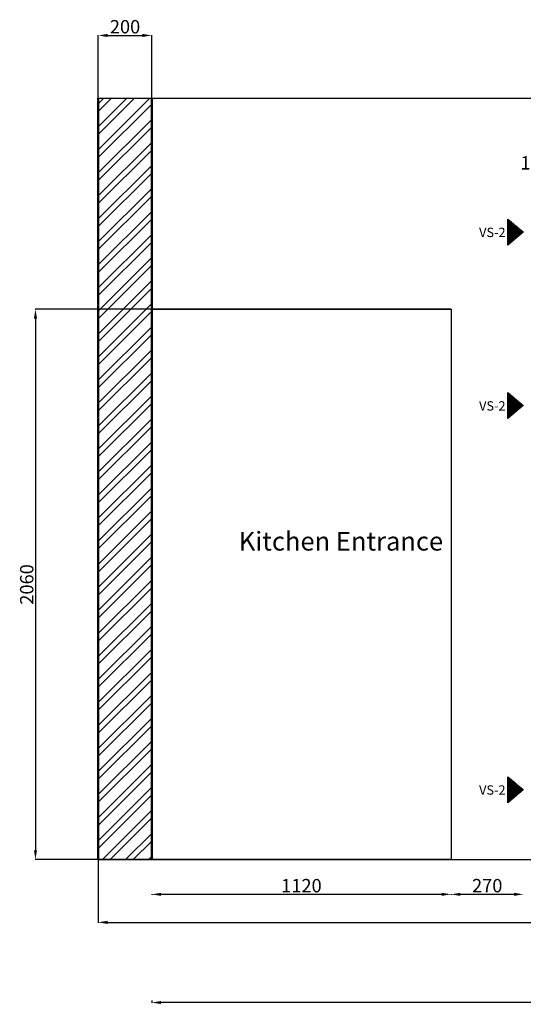
# Model space of a CAD drawing. Units: millimetres. Extents: x 407065 to 421840, y 1168257 to 1177792.
# Tile 11 of 17: x 413867 to 415751, y 1168495 to 1172181. Entities that reach past the tile are written whole.
import ezdxf

# ---------------------------------------------------------------- set-up
doc = ezdxf.new("R2010")
doc.units = ezdxf.units.MM
for name, color, linetype, lineweight in [('A-ANNO-DIMS', 6, 'Continuous', 18), ('A-ANNO-TEXT', 30, 'Continuous', 18), ('A-FURN', 3, 'Continuous', 25), ('A-WALL', 7, 'Continuous', 50), ('A-WALL-PATT', 8, 'Continuous', 13)]:
    doc.layers.add(name, color=color, linetype=linetype, lineweight=lineweight)
doc.styles.get("Standard").update_dxf_attribs({"font": 'arial.ttf'})
doc.dimstyles.new('ISO-25', dxfattribs={"dimtxt": 50, "dimasz": 35, "dimexe": 1.25, "dimexo": 0.625, "dimtad": 1, "dimdec": 1, "dimtxsty": 'Standard', "dimcen": 35, "dimadec": 0, "dimazin": 0, "dimtfac": 1, "dimtdec": 1, "dimtmove": 0, "dimatfit": 3, "dimfxl": 1, "dimarcsym": 0})

# ---------------------------------------------------------------- blocks, each defined once
blk = doc.blocks.new('*D154')
at = {"layer": 'A-ANNO-DIMS', "color": 0, "lineweight": -2, "transparency": 16777216}
for p, q in [((415480.9, 1168907.3), (415480.9, 1168907.9)), ((415715.9, 1168906.7), (415515.9, 1168906.7)), ((415750.9, 1168907.3), (415750.9, 1168907.9))]:
    blk.add_line(p, q, dxfattribs=at)
at = {"layer": 'A-ANNO-DIMS', "color": 0, "transparency": 16777216}
for points in [[(415515.9, 1168912.5), (415515.9, 1168900.9), (415480.9, 1168906.7)], [(415715.9, 1168912.5), (415715.9, 1168900.9), (415750.9, 1168906.7)]]:
    blk.add_solid(points, dxfattribs=at)
at = {"layer": 'Defpoints', "color": 0, "transparency": 16777216}
for p in [(415480.9, 1168906.7), (415480.9, 1168906.7), (415750.9, 1168906.7)]:
    blk.add_point(p, dxfattribs=at)
at = {"layer": 'A-ANNO-DIMS', "color": 0, "transparency": 16777216, "insert": (415615.9, 1168932.8), "char_height": 50, "attachment_point": 5}
blk.add_mtext('270', dxfattribs=at)
blk = doc.blocks.new('*D155')
at = {"layer": 'A-ANNO-DIMS', "color": 0, "lineweight": -2, "transparency": 16777216}
for p, q in [((414360.9, 1168907.3), (414360.9, 1168905.4)), ((415445.9, 1168906.7), (414395.9, 1168906.7)), ((415480.9, 1168907.3), (415480.9, 1168905.4))]:
    blk.add_line(p, q, dxfattribs=at)
at = {"layer": 'A-ANNO-DIMS', "color": 0, "transparency": 16777216}
for points in [[(414395.9, 1168912.5), (414395.9, 1168900.9), (414360.9, 1168906.7)], [(415445.9, 1168912.5), (415445.9, 1168900.9), (415480.9, 1168906.7)]]:
    blk.add_solid(points, dxfattribs=at)
at = {"layer": 'Defpoints', "color": 0, "transparency": 16777216}
for p in [(414360.9, 1168907.9), (414360.9, 1168906.7), (415480.9, 1168907.9)]:
    blk.add_point(p, dxfattribs=at)
at = {"layer": 'A-ANNO-DIMS', "color": 0, "transparency": 16777216, "insert": (414920.9, 1168932.8), "char_height": 50, "attachment_point": 5}
blk.add_mtext('1120', dxfattribs=at)
blk = doc.blocks.new('*D158')
at = {"layer": 'A-ANNO-DIMS', "color": 0, "lineweight": -2, "transparency": 16777216}
for p, q in [((414360.9, 1168509.6), (414360.9, 1168500.5)), ((418115.9, 1168501.7), (414395.9, 1168501.7)), ((418150.9, 1168509.6), (418150.9, 1168500.5))]:
    blk.add_line(p, q, dxfattribs=at)
at = {"layer": 'A-ANNO-DIMS', "color": 0, "transparency": 16777216}
for points in [[(414395.9, 1168507.5), (414395.9, 1168495.9), (414360.9, 1168501.7)], [(418115.9, 1168507.5), (418115.9, 1168495.9), (418150.9, 1168501.7)]]:
    blk.add_solid(points, dxfattribs=at)
at = {"layer": 'Defpoints', "color": 0, "transparency": 16777216}
for p in [(414360.9, 1168510.3), (414360.9, 1168501.7), (418150.9, 1168510.3)]:
    blk.add_point(p, dxfattribs=at)
at = {"layer": 'A-ANNO-DIMS', "color": 0, "transparency": 16777216, "insert": (416255.9, 1168527.9), "char_height": 50, "attachment_point": 5}
blk.add_mtext('3790', dxfattribs=at)
blk = doc.blocks.new('SHUTTER-HANDLE-MARK')
h = blk.add_hatch()
h.set_pattern_fill('ANSI32', color=256, scale=0.08)
h.set_pattern_definition([(45, (-3404.92366, -221.627), (-0.53881536726, 0.53881536726), []), (45, (-3404.56445, -221.627), (-0.53881536726, 0.53881536726), [])])
h.paths.add_polyline_path([(420059.2, 1176549.9), (420001.3, 1176501.2), (420059.2, 1176452.5)])
h = blk.add_hatch(color=256)
h.dxf.hatch_style = 1
h.paths.add_polyline_path([(420059.2, 1176549.9), (420001.3, 1176501.2), (420059.2, 1176452.5)])
blk = doc.blocks.new('*D219')
at = {"layer": 'A-ANNO-DIMS', "color": 0, "lineweight": -2, "transparency": 16777216}
for p, q in [((414160.9, 1169036.2), (414160.9, 1168800.6)), ((418450.9, 1169036.2), (418450.9, 1168800.6)), ((414195.9, 1168801.8), (418415.9, 1168801.8))]:
    blk.add_line(p, q, dxfattribs=at)
at = {"layer": 'A-ANNO-DIMS', "color": 0, "transparency": 16777216}
for points in [[(414195.9, 1168807.7), (414195.9, 1168796), (414160.9, 1168801.8)], [(418415.9, 1168807.7), (418415.9, 1168796), (418450.9, 1168801.8)]]:
    blk.add_solid(points, dxfattribs=at)
at = {"layer": 'Defpoints', "color": 0, "transparency": 16777216}
for p in [(414160.9, 1169036.8), (418450.9, 1169036.8), (418450.9, 1168801.8)]:
    blk.add_point(p, dxfattribs=at)
at = {"layer": 'A-ANNO-DIMS', "color": 0, "transparency": 16777216, "insert": (416305.9, 1168828), "char_height": 50, "attachment_point": 5}
blk.add_mtext('4290', dxfattribs=at)
blk = doc.blocks.new('*D220')
at = {"layer": 'A-ANNO-DIMS', "color": 0, "lineweight": -2, "transparency": 16777216}
for p, q in [((414160.9, 1171887.4), (414160.9, 1172123.1)), ((414195.9, 1172121.8), (414325.9, 1172121.8)), ((414360.9, 1171887.4), (414360.9, 1172123.1))]:
    blk.add_line(p, q, dxfattribs=at)
at = {"layer": 'A-ANNO-DIMS', "color": 0, "transparency": 16777216}
for points in [[(414195.9, 1172127.7), (414195.9, 1172116), (414160.9, 1172121.8)], [(414325.9, 1172127.7), (414325.9, 1172116), (414360.9, 1172121.8)]]:
    blk.add_solid(points, dxfattribs=at)
at = {"layer": 'Defpoints', "color": 0, "transparency": 16777216}
for p in [(414360.9, 1172121.8), (414160.9, 1171886.8), (414360.9, 1171886.8)]:
    blk.add_point(p, dxfattribs=at)
at = {"layer": 'A-ANNO-DIMS', "color": 0, "transparency": 16777216, "insert": (414260.9, 1172148), "char_height": 50, "attachment_point": 5}
blk.add_mtext('200', dxfattribs=at)
blk = doc.blocks.new('*D222')
at = {"layer": 'A-ANNO-DIMS', "color": 0, "lineweight": -2, "transparency": 16777216}
for p, q in [((415480.2, 1171096.8), (413924.6, 1171096.8)), ((413925.9, 1171061.8), (413925.9, 1169071.8)), ((415480.2, 1169036.8), (413924.6, 1169036.8))]:
    blk.add_line(p, q, dxfattribs=at)
at = {"layer": 'A-ANNO-DIMS', "color": 0, "transparency": 16777216}
for points in [[(413920, 1171061.8), (413931.7, 1171061.8), (413925.9, 1171096.8)], [(413920, 1169071.8), (413931.7, 1169071.8), (413925.9, 1169036.8)]]:
    blk.add_solid(points, dxfattribs=at)
at = {"layer": 'Defpoints', "color": 0, "transparency": 16777216}
for p in [(415480.9, 1171096.8), (413925.9, 1169036.8), (415480.9, 1169036.8)]:
    blk.add_point(p, dxfattribs=at)
at = {"layer": 'A-ANNO-DIMS', "color": 0, "transparency": 16777216, "insert": (413899.7, 1170066.8), "char_height": 50, "attachment_point": 5, "rotation": 90}
blk.add_mtext('2060', dxfattribs=at)

msp = doc.modelspace()

# ---------------------------------------------------------------- hatches: boundary and pattern name
at = {"layer": 'A-WALL-PATT'}
h = msp.add_hatch(dxfattribs=at)
h.set_pattern_fill('ANSI32', color=256, scale=6.4, angle=180)
h.set_pattern_definition([(225, (-18706.866, -112.55), (43.1052294, -43.1052294), []), (225, (-18735.6, -112.55), (43.1052294, -43.1052294), [])])
h.paths.add_polyline_path([(414360.8552, 1171886.8201), (414160.8552, 1171886.8201), (414160.8552, 1169036.8201), (414360.8552, 1169036.8201)])

# ---------------------------------------------------------------- linework, layer by layer
at = {"layer": 'A-FURN'}
for p, q in [((414160.8552, 1171886.8201), (418450.8552, 1171886.8201)), ((414360.8552, 1171096.8201), (415480.8552, 1171096.8201)), ((415480.8552, 1171096.8201), (415480.8552, 1169036.8201)), ((414160.8552, 1169036.8201), (418450.8552, 1169036.8201))]:
    msp.add_line(p, q, dxfattribs=at)
for points in [[(415692.9322, 1171434.2902), (415750.8552, 1171385.6064), (415692.9322, 1171336.9226)], [(415692.9322, 1170784.6991), (415750.8552, 1170736.0153), (415692.9322, 1170687.3315)], [(415692.9322, 1169346.8751), (415750.8552, 1169298.1913), (415692.9322, 1169249.5075)]]:
    msp.add_lwpolyline(points, close=True, dxfattribs=at)
at = {"layer": 'A-WALL'}
for p, q in [((414160.8552, 1171886.8201), (414160.8552, 1169036.8201)), ((414360.8552, 1171886.8201), (414360.8552, 1169036.8201))]:
    msp.add_line(p, q, dxfattribs=at)

# ---------------------------------------------------------------- block references
at = {"layer": 'A-FURN', "extrusion": (0, 0, -1), "zscale": -1}
for p in [(-835752.1322, -5115.5619), (-835752.1322, -5765.153), (-835752.1322, -7202.9769)]:
    msp.add_blockref('SHUTTER-HANDLE-MARK', p, dxfattribs=at)

# ---------------------------------------------------------------- texts
at = {"layer": 'A-ANNO-TEXT'}
for s, width, insert, char_height, attachment_point in [(' 1-Openable Shutter', 721.424123, (415724.6749, 1171670.0044), 50, 1), ('VS-2', 382.409863, (415684.4691, 1171402.1059), 35, 3), ('VS-2', 382.409863, (415684.4691, 1170752.5148), 35, 3), ('Kitchen Entrance', 785.351562, (414686.4619, 1170263.5723), 70, 1), ('VS-2', 382.409863, (415684.4691, 1169314.6909), 35, 3)]:
    msp.add_mtext_dynamic_manual_height_columns(s, width=width, gutter_width=12.5, heights=[0], dxfattribs=dict(at, insert=insert, char_height=char_height, attachment_point=attachment_point))

# ---------------------------------------------------------------- dimensions: what is measured, and where the dimension line sits
at = {"layer": 'A-ANNO-DIMS'}
for base, p1, p2, override, picture, middle in [((414360.8552, 1172121.8201), (414160.8552, 1171886.8201), (414360.8552, 1171886.8201), {"dimdec": 0, "dimlfac": 1, "dimrnd": 0, "dimzin": 0, "dimdsep": 46, "dimlunit": 2}, '*D220', (414260.8552, 1172147.9738)), ((418450.8552, 1168801.8201), (414160.8552, 1169036.8201), (418450.8552, 1169036.8201), {"dimdec": 0, "dimlfac": 1, "dimrnd": 0, "dimzin": 0, "dimdsep": 46, "dimlunit": 2}, '*D219', (416305.8552, 1168827.9738)), ((414360.8552, 1168906.6929), (415480.8552, 1168907.9429), (414360.8552, 1168907.9429), {"dimclrd": 0, "dimclre": 0, "dimclrt": 0}, '*D155', (414920.8552, 1168932.8466)), ((415480.8552, 1168906.6929), (415750.8552, 1168906.6929), (415480.8552, 1168906.6929), {"dimclrd": 0, "dimclre": 0, "dimclrt": 0}, '*D154', (415615.8552, 1168932.8466)), ((414360.8552, 1168501.7014), (418150.8552, 1168510.2523), (414360.8552, 1168510.2523), {"dimclrd": 0, "dimclre": 0, "dimclrt": 0}, '*D158', (416255.8552, 1168527.8721))]:
    dim = msp.add_linear_dim(base=base, p1=p1, p2=p2, dimstyle='ISO-25', override=override, dxfattribs=at)
    dim.commit()
    dim.dimension.update_dxf_attribs({"geometry": picture, "text_midpoint": middle})
dim = msp.add_linear_dim(base=(413925.8552, 1169036.8201), p1=(415480.8552, 1171096.8201), p2=(415480.8552, 1169036.8201), angle=90, dimstyle='ISO-25', override={"dimdec": 0, "dimlfac": 1, "dimrnd": 0, "dimzin": 0, "dimdsep": 46, "dimlunit": 2}, dxfattribs=at)
dim.commit()
dim.dimension.update_dxf_attribs({"geometry": '*D222', "text_midpoint": (413899.7015, 1170066.8201)})

doc.saveas('drawing.dxf')
